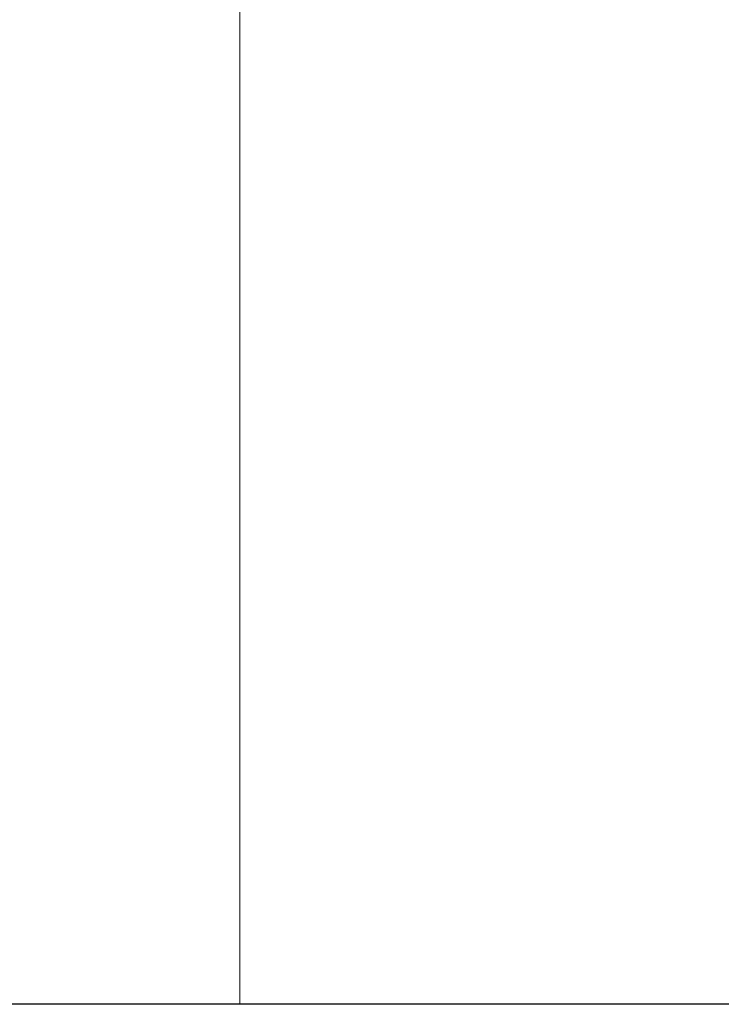
# Model space of a CAD drawing. Units: inches. Extents: x 2091 to 2899, y 967 to 2217.
# Tile 161 of 256: x 2203.1037 to 2203.14205, y 1152.24706 to 1152.30086. Entities that reach past the tile are written whole.
import ezdxf

# ---------------------------------------------------------------- set-up
doc = ezdxf.new("R2010")
doc.units = ezdxf.units.IN
doc.layers.add('A-ANNO-DIMS', color=2, linetype='Continuous', lineweight=18)
doc.layers.add('A-GLAZ', color=4, linetype='Continuous', lineweight=18)
doc.styles.get("Standard").update_dxf_attribs({"font": 'arial.ttf'})
doc.dimstyles.new('ISO-25', dxfattribs={"dimtxt": 4, "dimasz": 4, "dimexe": 1.25, "dimexo": 0.625, "dimtad": 1, "dimdec": 0, "dimlunit": 3, "dimtxsty": 'Standard', "dimcen": 2.5, "dimadec": 0, "dimazin": 0, "dimtfac": 1, "dimtdec": 0, "dimtmove": 0, "dimatfit": 3, "dimfxl": 1, "dimarcsym": 0})

# ---------------------------------------------------------------- blocks, each defined once
blk = doc.blocks.new('WIN-DOUBLE-LINE')
for p, q in [((0.000398, -0.000445), (0.000398, 80.8229)), ((9.160288, -0.000445), (0.000398, -0.000445))]:
    blk.add_line(p, q)
blk = doc.blocks.new('*D91')
at = {"layer": 'A-ANNO-DIMS', "color": 0, "lineweight": -2, "transparency": 16777216}
for p, q in [((2211.650633, 1152.24706), (2098.311334, 1152.24706)), ((2099.561334, 1103.919059), (2099.561334, 1148.24706)), ((2211.518603, 1099.919059), (2098.311334, 1099.919059))]:
    blk.add_line(p, q, dxfattribs=at)
at = {"layer": 'A-ANNO-DIMS', "color": 0, "transparency": 16777216}
for points in [[(2098.894667, 1148.24706), (2100.228001, 1148.24706), (2099.561334, 1152.24706)], [(2098.894667, 1103.919059), (2100.228001, 1103.919059), (2099.561334, 1099.919059)]]:
    blk.add_solid(points, dxfattribs=at)
at = {"layer": 'Defpoints', "color": 0, "transparency": 16777216}
for p in [(2099.561334, 1152.24706), (2212.275633, 1152.24706), (2212.143603, 1099.919059)]:
    blk.add_point(p, dxfattribs=at)
at = {"layer": 'A-ANNO-DIMS', "color": 0, "transparency": 16777216, "insert": (2096.868121, 1126.083059), "char_height": 4, "attachment_point": 5, "rotation": 90}
blk.add_mtext('4\'-4 1/2"', dxfattribs=at)

msp = doc.modelspace()

# ---------------------------------------------------------------- block references
at = {"layer": 'A-GLAZ'}
msp.add_blockref('WIN-DOUBLE-LINE', (2203.115344, 1152.247505), dxfattribs=at)

# ---------------------------------------------------------------- dimensions: what is measured, and where the dimension line sits
at = {"layer": 'A-ANNO-DIMS'}
dim = msp.add_linear_dim(base=(2099.561334, 1152.24706), p1=(2212.143603, 1099.919059), p2=(2212.275633, 1152.24706), angle=90, dimstyle='ISO-25', override={"dimdec": 1, "dimlfac": 1, "dimrnd": 0, "dimzin": 1, "dimdsep": 46, "dimlunit": 4, "dimfrac": 2}, dxfattribs=at)
dim.commit()
dim.dimension.update_dxf_attribs({"geometry": '*D91', "text_midpoint": (2096.868121, 1126.083059)})

doc.saveas('drawing.dxf')
